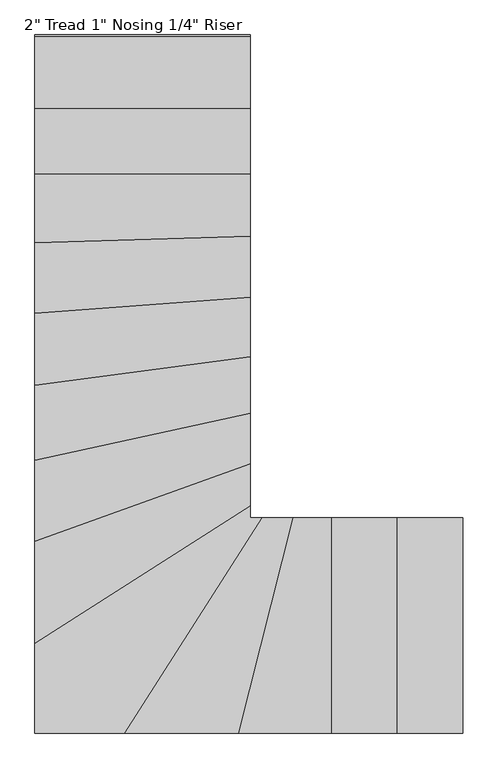
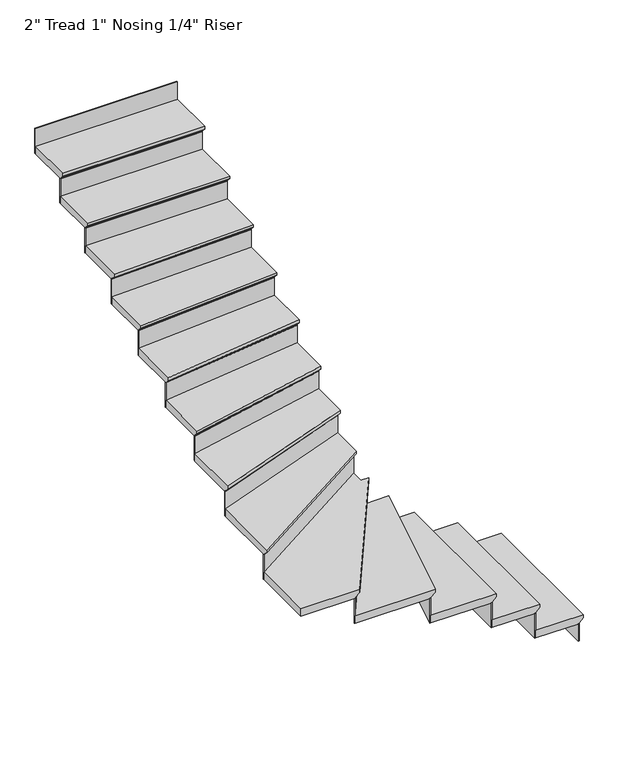
"""IFC4 building model written with IfcOpenShell, lengths in millimetres: stair flight geometry."""

from ifc_helpers import new_model, si_unit, origin, place, context, project, spatial, faceted_brep, source, transform, mapped, element, save


def stair_flight_62476df0(model_context):
    return source(origin(), model_context, "Body", "Brep", [
        faceted_brep([(-4378.4230036, -1246.1564015, 7228.4166667), (-4378.4230036, -1246.1564015, 7247.4666667), (-4378.4230036, -2160.5564015, 7247.4666667), (-4378.4230036, -2160.5564015, 7228.4166667), (-4403.8230036, -1246.1564015, 7203.0166667), (-4403.8230036, -2160.5564015, 7203.0166667), (-4683.2230036, -1246.1564015, 7247.4666667), (-4683.2230036, -2160.5564015, 7247.4666667), (-4403.8230036, -2160.5564015, 7196.6666667), (-4683.2230036, -2160.5564015, 7196.6666667), (-4683.2230036, -1246.1564015, 7196.6666667), (-4403.8230036, -1246.1564015, 7196.6666667)], [[[0, 1, 2, 3]], [[4, 0, 3, 5]], [[2, 1, 6, 7]], [[8, 9, 10, 11]], [[2, 7, 9, 8, 5, 3]], [[8, 11, 4, 5]], [[6, 1, 0, 4, 11, 10]], [[7, 6, 10, 9]]]),
        faceted_brep([(-4403.8230036, -1246.1564015, 7196.6666667), (-4403.8230036, -1246.1564015, 7078.1333333), (-4410.1730036, -1246.1564015, 7078.1333333), (-4410.1730036, -1246.1564015, 7196.6666667), (-4403.8230036, -2160.5564015, 7196.6666667), (-4410.1730036, -2160.5564015, 7196.6666667), (-4410.1730036, -2160.5564015, 7078.1333333), (-4403.8230036, -2160.5564015, 7078.1333333)], [[[0, 1, 2, 3]], [[4, 5, 6, 7]], [[1, 0, 4, 7]], [[2, 1, 7, 6]], [[3, 2, 6, 5]], [[0, 3, 5, 4]]]),
        faceted_brep([(-4683.2230036, -1246.1564015, 7366.0), (-4683.2230036, -1246.1564015, 7196.6666667), (-4689.5730036, -1246.1564015, 7196.6666667), (-4689.5730036, -1246.1564015, 7366.0), (-4683.2230036, -2160.5564015, 7366.0), (-4689.5730036, -2160.5564015, 7366.0), (-4689.5730036, -2160.5564015, 7196.6666667), (-4683.2230036, -2160.5564015, 7196.6666667)], [[[0, 1, 2, 3]], [[4, 5, 6, 7]], [[1, 0, 4, 7]], [[2, 1, 7, 6]], [[3, 2, 6, 5]], [[0, 3, 5, 4]]]),
        faceted_brep([(-4657.8230036, -2160.5564015, 7416.8), (-4657.8230036, -1246.1564015, 7416.8), (-4962.6230036, -1246.1564015, 7416.8), (-4962.6230036, -2160.5564015, 7416.8), (-4683.2230036, -2160.5564015, 7366.0), (-4962.6230036, -2160.5564015, 7366.0), (-4962.6230036, -1246.1564015, 7366.0), (-4683.2230036, -1246.1564015, 7366.0), (-4683.2230036, -2160.5564015, 7372.35), (-4657.8230036, -2160.5564015, 7397.75), (-4683.2230036, -1246.1564015, 7372.35), (-4657.8230036, -1246.1564015, 7397.75)], [[[0, 1, 2, 3]], [[4, 5, 6, 7]], [[0, 3, 5, 4, 8, 9]], [[4, 7, 10, 8]], [[2, 1, 11, 10, 7, 6]], [[3, 2, 6, 5]], [[11, 1, 0, 9]], [[10, 11, 9, 8]]]),
        faceted_brep([(-4962.6230036, -1246.1564015, 7535.3333333), (-4962.6230036, -1246.1564015, 7366.0), (-4968.9730036, -1246.1564015, 7366.0), (-4968.9730036, -1246.1564015, 7535.3333333), (-4962.6230036, -2160.5564015, 7535.3333333), (-4968.9730036, -2160.5564015, 7535.3333333), (-4968.9730036, -2160.5564015, 7366.0), (-4962.6230036, -2160.5564015, 7366.0)], [[[0, 1, 2, 3]], [[4, 5, 6, 7]], [[1, 0, 4, 7]], [[2, 1, 7, 6]], [[3, 2, 6, 5]], [[0, 3, 5, 4]]]),
        faceted_brep([(-4937.2230036, -2160.5564015, 7586.1333333), (-4937.2230036, -1246.1564015, 7586.1333333), (-5127.3280374, -1246.1564015, 7586.1333333), (-5358.313714, -2160.5564015, 7586.1333333), (-4962.6230036, -2160.5564015, 7535.3333333), (-5358.313714, -2160.5564015, 7535.3333333), (-5127.3280374, -1246.1564015, 7535.3333333), (-4962.6230036, -1246.1564015, 7535.3333333), (-4962.6230036, -2160.5564015, 7541.6833333), (-4937.2230036, -2160.5564015, 7567.0833333), (-4962.6230036, -1246.1564015, 7541.6833333), (-4937.2230036, -1246.1564015, 7567.0833333)], [[[0, 1, 2, 3]], [[4, 5, 6, 7]], [[0, 3, 5, 4, 8, 9]], [[4, 7, 10, 8]], [[2, 1, 11, 10, 7, 6]], [[3, 2, 6, 5]], [[11, 1, 0, 9]], [[10, 11, 9, 8]]]),
        faceted_brep([(-5127.3280374, -1246.1564015, 7704.6666667), (-5127.3280374, -1246.1564015, 7535.3333333), (-5133.8775055, -1246.1564015, 7535.3333333), (-5133.8775055, -1246.1564015, 7704.6666667), (-5358.313714, -2160.5564015, 7704.6666667), (-5364.8631821, -2160.5564015, 7704.6666667), (-5364.8631821, -2160.5564015, 7535.3333333), (-5358.313714, -2160.5564015, 7535.3333333)], [[[0, 1, 2, 3]], [[4, 5, 6, 7]], [[1, 0, 4, 7]], [[2, 1, 7, 6]], [[3, 2, 6, 5]], [[0, 3, 5, 4]]]),
        faceted_brep([(-5332.1158419, -2160.5564015, 7755.4666667), (-5101.1301653, -1246.1564015, 7755.4666667), (-5261.5956265, -1246.1564015, 7755.4666667), (-5846.1950619, -2160.5564015, 7755.4666667), (-5358.313714, -2160.5564015, 7704.6666667), (-5846.1950619, -2160.5564015, 7704.6666667), (-5261.5956265, -1246.1564015, 7704.6666667), (-5127.3280374, -1246.1564015, 7704.6666667), (-5358.313714, -2160.5564015, 7711.0166667), (-5332.1158419, -2160.5564015, 7736.4166667), (-5127.3280374, -1246.1564015, 7711.0166667), (-5101.1301653, -1246.1564015, 7736.4166667)], [[[0, 1, 2, 3]], [[4, 5, 6, 7]], [[0, 3, 5, 4, 8, 9]], [[4, 7, 10, 8]], [[2, 1, 11, 10, 7, 6]], [[3, 2, 6, 5]], [[11, 1, 0, 9]], [[10, 11, 9, 8]]]),
        faceted_brep([(-5261.5956265, -1246.1564015, 7874.0), (-5261.5956265, -1246.1564015, 7704.6666667), (-5269.1324569, -1246.1564015, 7704.6666667), (-5269.1324569, -1246.1564015, 7874.0), (-5846.1950619, -2160.5564015, 7874.0), (-5853.7318923, -2160.5564015, 7874.0), (-5853.7318923, -2160.5564015, 7704.6666667), (-5846.1950619, -2160.5564015, 7704.6666667)], [[[0, 1, 2, 3]], [[4, 5, 6, 7]], [[1, 0, 4, 7]], [[2, 1, 7, 6]], [[3, 2, 6, 5]], [[0, 3, 5, 4]]]),
        faceted_brep([(-6196.7599931, -1749.696827, 7924.8), (-6196.7599931, -2160.5564015, 7924.8), (-5816.0477402, -2160.5564015, 7924.8), (-5231.4483048, -1246.1564015, 7924.8), (-5282.3599931, -1246.1564015, 7924.8), (-5282.3599931, -1165.0973916, 7924.8), (-6196.7599931, -2160.5564015, 7874.0), (-6196.7599931, -1749.696827, 7874.0), (-5282.3599931, -1165.0973916, 7874.0), (-5282.3599931, -1246.1564015, 7874.0), (-5261.5956265, -1246.1564015, 7874.0), (-5846.1950619, -2160.5564015, 7874.0), (-5261.5956265, -1246.1564015, 7880.35), (-5846.1950619, -2160.5564015, 7880.35), (-5231.4483048, -1246.1564015, 7905.75), (-5816.0477402, -2160.5564015, 7905.75)], [[[0, 1, 2, 3, 4, 5]], [[6, 7, 8, 9, 10, 11]], [[1, 0, 7, 6]], [[11, 10, 12, 13]], [[4, 3, 14, 12, 10, 9]], [[0, 5, 8, 7]], [[14, 3, 2, 15]], [[12, 14, 15, 13]], [[2, 1, 6, 11, 13, 15]], [[5, 4, 9, 8]]]),
        faceted_brep([(-5282.3599931, -1165.0973916, 8043.3333333), (-5282.3599931, -1165.0973916, 7874.0), (-5282.3599931, -1157.5605612, 7874.0), (-5282.3599931, -1157.5605612, 8043.3333333), (-6196.7599931, -1749.696827, 8043.3333333), (-6196.7599931, -1742.1599966, 8043.3333333), (-6196.7599931, -1742.1599966, 7874.0), (-6196.7599931, -1749.696827, 7874.0)], [[[0, 1, 2, 3]], [[4, 5, 6, 7]], [[1, 0, 4, 7]], [[2, 1, 7, 6]], [[3, 2, 6, 5]], [[0, 3, 5, 4]]]),
        faceted_brep([(-6196.7599931, -1779.8441487, 8094.1333333), (-5282.3599931, -1195.2447133, 8094.1333333), (-5282.3599931, -989.1410797, 8094.1333333), (-6196.7599931, -1317.7175845, 8094.1333333), (-6196.7599931, -1749.696827, 8043.3333333), (-6196.7599931, -1317.7175845, 8043.3333333), (-5282.3599931, -989.1410797, 8043.3333333), (-5282.3599931, -1165.0973916, 8043.3333333), (-6196.7599931, -1749.696827, 8049.6833333), (-6196.7599931, -1779.8441487, 8075.0833333), (-5282.3599931, -1165.0973916, 8049.6833333), (-5282.3599931, -1195.2447133, 8075.0833333)], [[[0, 1, 2, 3]], [[4, 5, 6, 7]], [[0, 3, 5, 4, 8, 9]], [[4, 7, 10, 8]], [[2, 1, 11, 10, 7, 6]], [[3, 2, 6, 5]], [[11, 1, 0, 9]], [[10, 11, 9, 8]]]),
        faceted_brep([(-5282.3599931, -989.1410797, 8212.6666667), (-5282.3599931, -989.1410797, 8043.3333333), (-5282.3599931, -982.3935597, 8043.3333333), (-5282.3599931, -982.3935597, 8212.6666667), (-6196.7599931, -1317.7175845, 8212.6666667), (-6196.7599931, -1310.9700645, 8212.6666667), (-6196.7599931, -1310.9700645, 8043.3333333), (-6196.7599931, -1317.7175845, 8043.3333333)], [[[0, 1, 2, 3]], [[4, 5, 6, 7]], [[1, 0, 4, 7]], [[2, 1, 7, 6]], [[3, 2, 6, 5]], [[0, 3, 5, 4]]]),
        faceted_brep([(-6196.7599931, -1344.7076644, 8263.4666667), (-5282.3599931, -1016.1311596, 8263.4666667), (-5282.3599931, -775.0246806, 8263.4666667), (-6196.7599931, -975.0133472, 8263.4666667), (-6196.7599931, -1317.7175845, 8212.6666667), (-6196.7599931, -975.0133472, 8212.6666667), (-5282.3599931, -775.0246806, 8212.6666667), (-5282.3599931, -989.1410797, 8212.6666667), (-6196.7599931, -1317.7175845, 8219.0166667), (-6196.7599931, -1344.7076644, 8244.4166667), (-5282.3599931, -989.1410797, 8219.0166667), (-5282.3599931, -1016.1311596, 8244.4166667)], [[[0, 1, 2, 3]], [[4, 5, 6, 7]], [[0, 3, 5, 4, 8, 9]], [[4, 7, 10, 8]], [[2, 1, 11, 10, 7, 6]], [[3, 2, 6, 5]], [[11, 1, 0, 9]], [[10, 11, 9, 8]]]),
        faceted_brep([(-5282.3599931, -775.0246806, 8382.0), (-5282.3599931, -775.0246806, 8212.6666667), (-5282.3599931, -768.5245811, 8212.6666667), (-5282.3599931, -768.5245811, 8382.0), (-6196.7599931, -975.0133472, 8382.0), (-6196.7599931, -968.5132477, 8382.0), (-6196.7599931, -968.5132477, 8212.6666667), (-6196.7599931, -975.0133472, 8212.6666667)], [[[0, 1, 2, 3]], [[4, 5, 6, 7]], [[1, 0, 4, 7]], [[2, 1, 7, 6]], [[3, 2, 6, 5]], [[0, 3, 5, 4]]]),
        faceted_brep([(-6196.7599931, -1001.0137453, 8432.8), (-5282.3599931, -801.0250787, 8432.8), (-5282.3599931, -535.4776405, 8432.8), (-6196.7599931, -656.5180526, 8432.8), (-6196.7599931, -975.0133472, 8382.0), (-6196.7599931, -656.5180526, 8382.0), (-5282.3599931, -535.4776405, 8382.0), (-5282.3599931, -775.0246806, 8382.0), (-6196.7599931, -975.0133472, 8388.35), (-6196.7599931, -1001.0137453, 8413.75), (-5282.3599931, -775.0246806, 8388.35), (-5282.3599931, -801.0250787, 8413.75)], [[[0, 1, 2, 3]], [[4, 5, 6, 7]], [[0, 3, 5, 4, 8, 9]], [[4, 7, 10, 8]], [[2, 1, 11, 10, 7, 6]], [[3, 2, 6, 5]], [[11, 1, 0, 9]], [[10, 11, 9, 8]]]),
        faceted_brep([(-5282.3599931, -535.4776405, 8551.3333333), (-5282.3599931, -535.4776405, 8382.0), (-5282.3599931, -529.0722492, 8382.0), (-5282.3599931, -529.0722492, 8551.3333333), (-6196.7599931, -656.5180526, 8551.3333333), (-6196.7599931, -650.1126613, 8551.3333333), (-6196.7599931, -650.1126613, 8382.0), (-6196.7599931, -656.5180526, 8382.0)], [[[0, 1, 2, 3]], [[4, 5, 6, 7]], [[1, 0, 4, 7]], [[2, 1, 7, 6]], [[3, 2, 6, 5]], [[0, 3, 5, 4]]]),
        faceted_brep([(-6196.7599931, -682.139618, 8602.1333333), (-5282.3599931, -561.099206, 8602.1333333), (-5282.3599931, -282.9309158, 8602.1333333), (-6196.7599931, -350.56912, 8602.1333333), (-6196.7599931, -656.5180526, 8551.3333333), (-6196.7599931, -350.56912, 8551.3333333), (-5282.3599931, -282.9309158, 8551.3333333), (-5282.3599931, -535.4776405, 8551.3333333), (-6196.7599931, -656.5180526, 8557.6833333), (-6196.7599931, -682.139618, 8583.0833333), (-5282.3599931, -535.4776405, 8557.6833333), (-5282.3599931, -561.099206, 8583.0833333)], [[[0, 1, 2, 3]], [[4, 5, 6, 7]], [[0, 3, 5, 4, 8, 9]], [[4, 7, 10, 8]], [[2, 1, 11, 10, 7, 6]], [[3, 2, 6, 5]], [[11, 1, 0, 9]], [[10, 11, 9, 8]]]),
        faceted_brep([(-5282.3599931, -282.9309158, 8720.6666667), (-5282.3599931, -282.9309158, 8551.3333333), (-5282.3599931, -276.5635673, 8551.3333333), (-5282.3599931, -276.5635673, 8720.6666667), (-6196.7599931, -350.56912, 8720.6666667), (-6196.7599931, -344.2017715, 8720.6666667), (-6196.7599931, -344.2017715, 8551.3333333), (-6196.7599931, -350.56912, 8551.3333333)], [[[0, 1, 2, 3]], [[4, 5, 6, 7]], [[1, 0, 4, 7]], [[2, 1, 7, 6]], [[3, 2, 6, 5]], [[0, 3, 5, 4]]]),
        faceted_brep([(-6196.7599931, -376.0385141, 8771.4666667), (-5282.3599931, -308.4003099, 8771.4666667), (-5282.3599931, -22.8518026, 8771.4666667), (-6196.7599931, -51.9612867, 8771.4666667), (-6196.7599931, -350.56912, 8720.6666667), (-6196.7599931, -51.9612867, 8720.6666667), (-5282.3599931, -22.8518026, 8720.6666667), (-5282.3599931, -282.9309158, 8720.6666667), (-6196.7599931, -350.56912, 8727.0166667), (-6196.7599931, -376.0385141, 8752.4166667), (-5282.3599931, -282.9309158, 8727.0166667), (-5282.3599931, -308.4003099, 8752.4166667)], [[[0, 1, 2, 3]], [[4, 5, 6, 7]], [[0, 3, 5, 4, 8, 9]], [[4, 7, 10, 8]], [[2, 1, 11, 10, 7, 6]], [[3, 2, 6, 5]], [[11, 1, 0, 9]], [[10, 11, 9, 8]]]),
        faceted_brep([(-5282.3599931, -22.8518026, 8890.0), (-5282.3599931, -22.8518026, 8720.6666667), (-5282.3599931, -16.4985857, 8720.6666667), (-5282.3599931, -16.4985857, 8890.0), (-6196.7599931, -51.9612867, 8890.0), (-6196.7599931, -45.6080698, 8890.0), (-6196.7599931, -45.6080698, 8720.6666667), (-6196.7599931, -51.9612867, 8720.6666667)], [[[0, 1, 2, 3]], [[4, 5, 6, 7]], [[1, 0, 4, 7]], [[2, 1, 7, 6]], [[3, 2, 6, 5]], [[0, 3, 5, 4]]]),
        faceted_brep([(-6196.7599931, -77.3741541, 8940.8), (-5282.3599931, -48.26467, 8940.8), (-5282.3599931, 241.980588, 8940.8), (-6196.7599931, 241.980588, 8940.8), (-6196.7599931, -51.9612867, 8890.0), (-6196.7599931, 241.980588, 8890.0), (-5282.3599931, 241.980588, 8890.0), (-5282.3599931, -22.8518026, 8890.0), (-6196.7599931, -51.9612867, 8896.35), (-6196.7599931, -77.3741541, 8921.75), (-5282.3599931, -22.8518026, 8896.35), (-5282.3599931, -48.26467, 8921.75)], [[[0, 1, 2, 3]], [[4, 5, 6, 7]], [[0, 3, 5, 4, 8, 9]], [[4, 7, 10, 8]], [[2, 1, 11, 10, 7, 6]], [[3, 2, 6, 5]], [[11, 1, 0, 9]], [[10, 11, 9, 8]]]),
        faceted_brep([(-5282.3599931, 241.980588, 9059.3333333), (-5282.3599931, 241.980588, 8890.0), (-5282.3599931, 248.330588, 8890.0), (-5282.3599931, 248.330588, 9059.3333333), (-6196.7599931, 241.980588, 9059.3333333), (-6196.7599931, 248.330588, 9059.3333333), (-6196.7599931, 248.330588, 8890.0), (-6196.7599931, 241.980588, 8890.0)], [[[0, 1, 2, 3]], [[4, 5, 6, 7]], [[1, 0, 4, 7]], [[2, 1, 7, 6]], [[3, 2, 6, 5]], [[0, 3, 5, 4]]]),
        faceted_brep([(-6196.7599931, 216.580588, 9110.1333333), (-5282.3599931, 216.580588, 9110.1333333), (-5282.3599931, 521.380588, 9110.1333333), (-6196.7599931, 521.380588, 9110.1333333), (-6196.7599931, 241.980588, 9059.3333333), (-6196.7599931, 521.380588, 9059.3333333), (-5282.3599931, 521.380588, 9059.3333333), (-5282.3599931, 241.980588, 9059.3333333), (-6196.7599931, 241.980588, 9065.6833333), (-6196.7599931, 216.580588, 9091.0833333), (-5282.3599931, 241.980588, 9065.6833333), (-5282.3599931, 216.580588, 9091.0833333)], [[[0, 1, 2, 3]], [[4, 5, 6, 7]], [[0, 3, 5, 4, 8, 9]], [[4, 7, 10, 8]], [[2, 1, 11, 10, 7, 6]], [[3, 2, 6, 5]], [[11, 1, 0, 9]], [[10, 11, 9, 8]]]),
        faceted_brep([(-5282.3599931, 521.380588, 9228.6666667), (-5282.3599931, 521.380588, 9059.3333333), (-5282.3599931, 527.730588, 9059.3333333), (-5282.3599931, 527.730588, 9228.6666667), (-6196.7599931, 521.380588, 9228.6666667), (-6196.7599931, 527.730588, 9228.6666667), (-6196.7599931, 527.730588, 9059.3333333), (-6196.7599931, 521.380588, 9059.3333333)], [[[0, 1, 2, 3]], [[4, 5, 6, 7]], [[1, 0, 4, 7]], [[2, 1, 7, 6]], [[3, 2, 6, 5]], [[0, 3, 5, 4]]]),
        faceted_brep([(-5282.3599931, 800.780588, 9398.0), (-5282.3599931, 800.780588, 9228.6666667), (-5282.3599931, 807.130588, 9228.6666667), (-5282.3599931, 807.130588, 9398.0), (-6196.7599931, 800.780588, 9398.0), (-6196.7599931, 807.130588, 9398.0), (-6196.7599931, 807.130588, 9228.6666667), (-6196.7599931, 800.780588, 9228.6666667)], [[[0, 1, 2, 3]], [[4, 5, 6, 7]], [[1, 0, 4, 7]], [[2, 1, 7, 6]], [[3, 2, 6, 5]], [[0, 3, 5, 4]]]),
        faceted_brep([(-6196.7599931, 495.980588, 9279.4666667), (-5282.3599931, 495.980588, 9279.4666667), (-5282.3599931, 800.780588, 9279.4666667), (-6196.7599931, 800.780588, 9279.4666667), (-6196.7599931, 521.380588, 9228.6666667), (-6196.7599931, 800.780588, 9228.6666667), (-5282.3599931, 800.780588, 9228.6666667), (-5282.3599931, 521.380588, 9228.6666667), (-6196.7599931, 521.380588, 9235.0166667), (-6196.7599931, 495.980588, 9260.4166667), (-5282.3599931, 521.380588, 9235.0166667), (-5282.3599931, 495.980588, 9260.4166667)], [[[0, 1, 2, 3]], [[4, 5, 6, 7]], [[0, 3, 5, 4, 8, 9]], [[4, 7, 10, 8]], [[2, 1, 11, 10, 7, 6]], [[3, 2, 6, 5]], [[11, 1, 0, 9]], [[10, 11, 9, 8]]]),
    ])


if __name__ == "__main__":
    model = new_model("IFC4")
    model_context = context("Model", 3, world=origin())
    ifc_project = project(units=[si_unit("LENGTHUNIT", "METRE", prefix="MILLI")], contexts=[model_context])
    site = spatial("IfcSite", under=ifc_project)
    building = spatial("IfcBuilding", under=site)
    placement = place(None, origin())
    stair_flight_shape = stair_flight_62476df0(model_context)
    element("IfcStairFlight", 1, ObjectType="2\" Tread 1\" Nosing 1/4\" Riser", at=placement, inside=building, context=model_context, shape_type="MappedRepresentation", body=[
        mapped(stair_flight_shape, transform((0.0, 0.0, 0.0), x_axis=(1.0, 0.0, 0.0), y_axis=(0.0, 1.0, 0.0), z_axis=(0.0, 0.0, 1.0))),
    ])
    save(model, "model.ifc")
